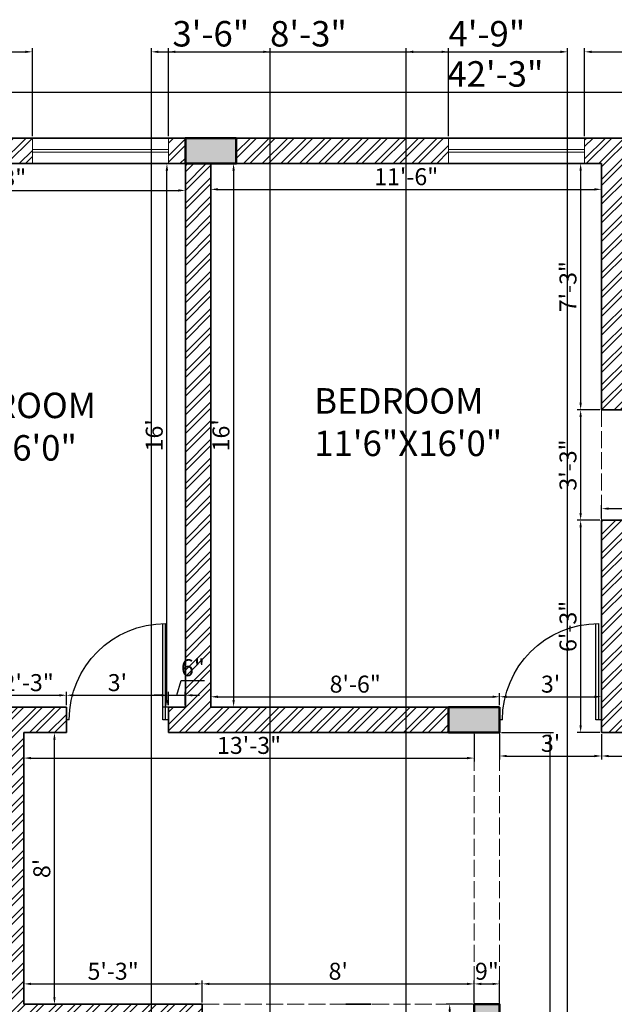
# Model space of a CAD drawing. Units: inches. Extents: x 4153 to 5577, y 785 to 1503.
# Tile 9 of 11: x 5097 to 5307, y 1138 to 1486. Entities that reach past the tile are written whole.
import ezdxf

# ---------------------------------------------------------------- set-up
doc = ezdxf.new("R2010")
doc.units = ezdxf.units.IN
doc.linetypes.add('ACAD_ISO02W100', pattern=[15, 12, -3])
for name, color, linetype, lineweight in [('A-ANNO-DIMS', 2, 'Continuous', 18), ('A-AREA-IDEN', 7, 'Continuous', 25), ('A-COLS', 7, 'Continuous', 50), ('A-DOOR', 3, 'Continuous', 25), ('A-GLAZ', 4, 'Continuous', 18), ('A-WALL', 7, 'Continuous', 35), ('A-WALL-OVHD', 7, 'ACAD_ISO02W100', 18)]:
    doc.layers.add(name, color=color, linetype=linetype, lineweight=lineweight)
doc.layers.add('A-WALL-PATT', color=251, linetype='Continuous', lineweight=13, true_color=0x636466)
doc.styles.get("Standard").update_dxf_attribs({"font": 'arial.ttf'})
doc.dimstyles.new('ISO-25', dxfattribs={"dimtxt": 9, "dimasz": 2.5, "dimexe": 1.25, "dimexo": 0.625, "dimtad": 1, "dimlunit": 3, "dimtxsty": 'Standard', "dimcen": 2.5, "dimadec": 0, "dimazin": 0, "dimtfac": 1, "dimtmove": 0, "dimatfit": 3, "dimfxl": 1, "dimarcsym": 0})

# ---------------------------------------------------------------- blocks, each defined once
blk = doc.blocks.new('D1')
for p, q in [((1, 0), (1, 34)), ((2, 0), (2, 33.99)), ((0, 0), (2, 0)), ((35, 0), (36, 0))]:
    blk.add_line(p, q)
at = {"ltscale": 0.5}
blk.add_arc((1, 0), 34, 0, 90, dxfattribs=at)
blk = doc.blocks.new('*D23')
at = {"layer": 'A-ANNO-DIMS', "color": 0, "lineweight": -2, "transparency": 16777216}
for p, q in [((5011.25, 1445.11), (5011.25, 1461.99)), ((5518.25, 1445.11), (5518.25, 1461.99)), ((5013.75, 1460.74), (5515.75, 1460.74))]:
    blk.add_line(p, q, dxfattribs=at)
at = {"layer": 'A-ANNO-DIMS', "color": 0, "transparency": 16777216}
for points in [[(5013.75, 1461.16), (5013.75, 1460.33), (5011.25, 1460.74)], [(5515.75, 1461.16), (5515.75, 1460.33), (5518.25, 1460.74)]]:
    blk.add_solid(points, dxfattribs=at)
at = {"layer": 'Defpoints', "color": 0, "transparency": 16777216}
for p in [(5518.25, 1460.74), (5011.25, 1444.49), (5518.25, 1444.49)]:
    blk.add_point(p, dxfattribs=at)
at = {"layer": 'A-ANNO-DIMS', "color": 0, "transparency": 16777216, "insert": (5264.75, 1465.97), "char_height": 9, "attachment_point": 5}
blk.add_mtext('42\'-3"', dxfattribs=at)
blk = doc.blocks.new('*D25')
at = {"layer": 'A-ANNO-DIMS', "color": 0, "lineweight": -2, "transparency": 16777216}
for p, q in [((5020.25, 1434.86), (5020.25, 1424.72)), ((5155.25, 1434.86), (5155.25, 1424.72)), ((5022.75, 1425.97), (5152.75, 1425.97))]:
    blk.add_line(p, q, dxfattribs=at)
at = {"layer": 'A-ANNO-DIMS', "color": 0, "transparency": 16777216}
for points in [[(5022.75, 1426.39), (5022.75, 1425.56), (5020.25, 1425.97)], [(5152.75, 1426.39), (5152.75, 1425.56), (5155.25, 1425.97)]]:
    blk.add_solid(points, dxfattribs=at)
at = {"layer": 'Defpoints', "color": 0, "transparency": 16777216}
for p in [(5020.25, 1435.49), (5155.25, 1435.49), (5155.25, 1425.97)]:
    blk.add_point(p, dxfattribs=at)
at = {"layer": 'A-ANNO-DIMS', "color": 0, "transparency": 16777216, "insert": (5087.75, 1429.66), "char_height": 6, "attachment_point": 5}
blk.add_mtext('11\'-3"', dxfattribs=at)
blk = doc.blocks.new('*D29')
at = {"layer": 'A-ANNO-DIMS', "color": 0, "lineweight": -2, "transparency": 16777216}
for p, q in [((5086.25, 1244.11), (5086.25, 1248.91)), ((5113.25, 1244.11), (5113.25, 1248.91)), ((5088.75, 1247.66), (5110.75, 1247.66))]:
    blk.add_line(p, q, dxfattribs=at)
at = {"layer": 'A-ANNO-DIMS', "color": 0, "transparency": 16777216}
for points in [[(5088.75, 1248.07), (5088.75, 1247.24), (5086.25, 1247.66)], [(5110.75, 1248.07), (5110.75, 1247.24), (5113.25, 1247.66)]]:
    blk.add_solid(points, dxfattribs=at)
at = {"layer": 'Defpoints', "color": 0, "transparency": 16777216}
for p in [(5113.25, 1247.66), (5086.25, 1243.49), (5113.25, 1243.49)]:
    blk.add_point(p, dxfattribs=at)
at = {"layer": 'A-ANNO-DIMS', "color": 0, "transparency": 16777216, "insert": (5099.75, 1251.35), "char_height": 6, "attachment_point": 5}
blk.add_mtext('2\'-3"', dxfattribs=at)
blk = doc.blocks.new('*D30')
at = {"layer": 'A-ANNO-DIMS', "color": 0, "lineweight": -2, "transparency": 16777216}
for p, q in [((5113.25, 1244.11), (5113.25, 1248.91)), ((5149.25, 1244.11), (5149.25, 1248.91)), ((5115.75, 1247.66), (5146.75, 1247.66))]:
    blk.add_line(p, q, dxfattribs=at)
at = {"layer": 'A-ANNO-DIMS', "color": 0, "transparency": 16777216}
for points in [[(5115.75, 1248.07), (5115.75, 1247.24), (5113.25, 1247.66)], [(5146.75, 1248.07), (5146.75, 1247.24), (5149.25, 1247.66)]]:
    blk.add_solid(points, dxfattribs=at)
at = {"layer": 'Defpoints', "color": 0, "transparency": 16777216}
for p in [(5149.25, 1247.66), (5113.25, 1243.49), (5149.25, 1243.49)]:
    blk.add_point(p, dxfattribs=at)
at = {"layer": 'A-ANNO-DIMS', "color": 0, "transparency": 16777216, "insert": (5131.25, 1251.35), "char_height": 6, "attachment_point": 5}
blk.add_mtext("3'", dxfattribs=at)
blk = doc.blocks.new('*D31')
at = {"layer": 'A-ANNO-DIMS', "color": 0, "lineweight": -2, "transparency": 16777216}
for p, q in [((5152.25, 1247.66), (5153.83, 1252.91)), ((5153.83, 1252.91), (5162.01, 1252.91)), ((5149.25, 1244.11), (5149.25, 1248.91)), ((5155.25, 1244.11), (5155.25, 1248.91)), ((5146.75, 1247.66), (5144.25, 1247.66)), ((5149.25, 1247.66), (5155.25, 1247.66)), ((5149.25, 1247.66), (5155.25, 1247.66)), ((5157.75, 1247.66), (5160.25, 1247.66))]:
    blk.add_line(p, q, dxfattribs=at)
at = {"layer": 'A-ANNO-DIMS', "color": 0, "transparency": 16777216}
for points in [[(5146.75, 1248.07), (5146.75, 1247.24), (5149.25, 1247.66)], [(5157.75, 1248.07), (5157.75, 1247.24), (5155.25, 1247.66)]]:
    blk.add_solid(points, dxfattribs=at)
at = {"layer": 'Defpoints', "color": 0, "transparency": 16777216}
for p in [(5155.25, 1247.66), (5149.25, 1243.49), (5155.25, 1243.49)]:
    blk.add_point(p, dxfattribs=at)
at = {"layer": 'A-ANNO-DIMS', "color": 0, "transparency": 16777216, "insert": (5157.92, 1256.6), "char_height": 6, "attachment_point": 5}
blk.add_mtext('6"', dxfattribs=at)
blk = doc.blocks.new('*D32')
at = {"layer": 'A-ANNO-DIMS', "color": 0, "lineweight": -2, "transparency": 16777216}
for p, q in [((5154.63, 1435.49), (5147.49, 1435.49)), ((5148.74, 1245.99), (5148.74, 1432.99)), ((5154.63, 1243.49), (5147.49, 1243.49))]:
    blk.add_line(p, q, dxfattribs=at)
at = {"layer": 'A-ANNO-DIMS', "color": 0, "transparency": 16777216}
for points in [[(5148.32, 1432.99), (5149.16, 1432.99), (5148.74, 1435.49)], [(5148.32, 1245.99), (5149.16, 1245.99), (5148.74, 1243.49)]]:
    blk.add_solid(points, dxfattribs=at)
at = {"layer": 'Defpoints', "color": 0, "transparency": 16777216}
for p in [(5148.74, 1435.49), (5155.25, 1435.49), (5155.25, 1243.49)]:
    blk.add_point(p, dxfattribs=at)
at = {"layer": 'A-ANNO-DIMS', "color": 0, "transparency": 16777216, "insert": (5145.05, 1339.49), "char_height": 6, "attachment_point": 5, "rotation": 90}
blk.add_mtext("16'", dxfattribs=at)
blk = doc.blocks.new('*D33')
at = {"layer": 'A-ANNO-DIMS', "color": 0, "lineweight": -2, "transparency": 16777216}
for p, q in [((5164.25, 1434.86), (5164.25, 1425.11)), ((5302.25, 1434.86), (5302.25, 1425.11)), ((5166.75, 1426.36), (5299.75, 1426.36))]:
    blk.add_line(p, q, dxfattribs=at)
at = {"layer": 'A-ANNO-DIMS', "color": 0, "transparency": 16777216}
for points in [[(5166.75, 1426.78), (5166.75, 1425.94), (5164.25, 1426.36)], [(5299.75, 1426.78), (5299.75, 1425.94), (5302.25, 1426.36)]]:
    blk.add_solid(points, dxfattribs=at)
at = {"layer": 'Defpoints', "color": 0, "transparency": 16777216}
for p in [(5164.25, 1435.49), (5302.25, 1435.49), (5302.25, 1426.36)]:
    blk.add_point(p, dxfattribs=at)
at = {"layer": 'A-ANNO-DIMS', "color": 0, "transparency": 16777216, "insert": (5233.25, 1430.05), "char_height": 6, "attachment_point": 5}
blk.add_mtext('11\'-6"', dxfattribs=at)
blk = doc.blocks.new('*D34')
at = {"layer": 'A-ANNO-DIMS', "color": 0, "lineweight": -2, "transparency": 16777216}
for p, q in [((5164.88, 1435.49), (5173.55, 1435.49)), ((5172.3, 1432.99), (5172.3, 1245.99)), ((5164.88, 1243.49), (5173.55, 1243.49))]:
    blk.add_line(p, q, dxfattribs=at)
at = {"layer": 'A-ANNO-DIMS', "color": 0, "transparency": 16777216}
for points in [[(5171.88, 1432.99), (5172.72, 1432.99), (5172.3, 1435.49)], [(5171.88, 1245.99), (5172.72, 1245.99), (5172.3, 1243.49)]]:
    blk.add_solid(points, dxfattribs=at)
at = {"layer": 'Defpoints', "color": 0, "transparency": 16777216}
for p in [(5164.25, 1435.49), (5164.25, 1243.49), (5172.3, 1243.49)]:
    blk.add_point(p, dxfattribs=at)
at = {"layer": 'A-ANNO-DIMS', "color": 0, "transparency": 16777216, "insert": (5168.61, 1339.49), "char_height": 6, "attachment_point": 5, "rotation": 90}
blk.add_mtext("16'", dxfattribs=at)
blk = doc.blocks.new('*D35')
at = {"layer": 'A-ANNO-DIMS', "color": 0, "lineweight": -2, "transparency": 16777216}
for p, q in [((5164.25, 1244.11), (5164.25, 1248.37)), ((5166.75, 1247.12), (5263.75, 1247.12)), ((5266.25, 1244.11), (5266.25, 1248.37))]:
    blk.add_line(p, q, dxfattribs=at)
at = {"layer": 'A-ANNO-DIMS', "color": 0, "transparency": 16777216}
for points in [[(5166.75, 1247.54), (5166.75, 1246.7), (5164.25, 1247.12)], [(5263.75, 1247.54), (5263.75, 1246.7), (5266.25, 1247.12)]]:
    blk.add_solid(points, dxfattribs=at)
at = {"layer": 'Defpoints', "color": 0, "transparency": 16777216}
for p in [(5266.25, 1247.12), (5164.25, 1243.49), (5266.25, 1243.49)]:
    blk.add_point(p, dxfattribs=at)
at = {"layer": 'A-ANNO-DIMS', "color": 0, "transparency": 16777216, "insert": (5215.25, 1250.81), "char_height": 6, "attachment_point": 5}
blk.add_mtext('8\'-6"', dxfattribs=at)
blk = doc.blocks.new('*D36')
at = {"layer": 'A-ANNO-DIMS', "color": 0, "lineweight": -2, "transparency": 16777216}
for p, q in [((5266.25, 1244.11), (5266.25, 1248.37)), ((5268.75, 1247.12), (5299.75, 1247.12)), ((5302.25, 1247.75), (5302.25, 1248.37))]:
    blk.add_line(p, q, dxfattribs=at)
at = {"layer": 'A-ANNO-DIMS', "color": 0, "transparency": 16777216}
for points in [[(5268.75, 1247.54), (5268.75, 1246.7), (5266.25, 1247.12)], [(5299.75, 1247.54), (5299.75, 1246.7), (5302.25, 1247.12)]]:
    blk.add_solid(points, dxfattribs=at)
at = {"layer": 'Defpoints', "color": 0, "transparency": 16777216}
for p in [(5302.25, 1247.12), (5302.25, 1247.12), (5266.25, 1243.49)]:
    blk.add_point(p, dxfattribs=at)
at = {"layer": 'A-ANNO-DIMS', "color": 0, "transparency": 16777216, "insert": (5284.25, 1250.81), "char_height": 6, "attachment_point": 5}
blk.add_mtext("3'", dxfattribs=at)
blk = doc.blocks.new('*D37')
at = {"layer": 'A-ANNO-DIMS', "color": 0, "lineweight": -2, "transparency": 16777216}
for p, q in [((5301.63, 1435.49), (5293.61, 1435.49)), ((5294.86, 1432.99), (5294.86, 1350.99)), ((5301.63, 1348.49), (5293.61, 1348.49))]:
    blk.add_line(p, q, dxfattribs=at)
at = {"layer": 'A-ANNO-DIMS', "color": 0, "transparency": 16777216}
for points in [[(5294.45, 1432.99), (5295.28, 1432.99), (5294.86, 1435.49)], [(5294.45, 1350.99), (5295.28, 1350.99), (5294.86, 1348.49)]]:
    blk.add_solid(points, dxfattribs=at)
at = {"layer": 'Defpoints', "color": 0, "transparency": 16777216}
for p in [(5302.25, 1435.49), (5294.86, 1348.49), (5302.25, 1348.49)]:
    blk.add_point(p, dxfattribs=at)
at = {"layer": 'A-ANNO-DIMS', "color": 0, "transparency": 16777216, "insert": (5291.17, 1391.99), "char_height": 6, "attachment_point": 5, "rotation": 90}
blk.add_mtext('7\'-3"', dxfattribs=at)
blk = doc.blocks.new('*D38')
at = {"layer": 'A-ANNO-DIMS', "color": 0, "lineweight": -2, "transparency": 16777216}
for p, q in [((5301.63, 1348.49), (5293.61, 1348.49)), ((5294.86, 1345.99), (5294.86, 1311.99)), ((5301.63, 1309.49), (5293.61, 1309.49))]:
    blk.add_line(p, q, dxfattribs=at)
at = {"layer": 'A-ANNO-DIMS', "color": 0, "transparency": 16777216}
for points in [[(5294.45, 1345.99), (5295.28, 1345.99), (5294.86, 1348.49)], [(5294.45, 1311.99), (5295.28, 1311.99), (5294.86, 1309.49)]]:
    blk.add_solid(points, dxfattribs=at)
at = {"layer": 'Defpoints', "color": 0, "transparency": 16777216}
for p in [(5302.25, 1348.49), (5294.86, 1309.49), (5302.25, 1309.49)]:
    blk.add_point(p, dxfattribs=at)
at = {"layer": 'A-ANNO-DIMS', "color": 0, "transparency": 16777216, "insert": (5291.17, 1328.99), "char_height": 6, "attachment_point": 5, "rotation": 90}
blk.add_mtext('3\'-3"', dxfattribs=at)
blk = doc.blocks.new('*D39')
at = {"layer": 'A-ANNO-DIMS', "color": 0, "lineweight": -2, "transparency": 16777216}
for p, q in [((5301.63, 1309.49), (5293.61, 1309.49)), ((5294.86, 1306.99), (5294.86, 1236.99)), ((5301.63, 1234.49), (5293.61, 1234.49))]:
    blk.add_line(p, q, dxfattribs=at)
at = {"layer": 'A-ANNO-DIMS', "color": 0, "transparency": 16777216}
for points in [[(5294.45, 1306.99), (5295.28, 1306.99), (5294.86, 1309.49)], [(5294.45, 1236.99), (5295.28, 1236.99), (5294.86, 1234.49)]]:
    blk.add_solid(points, dxfattribs=at)
at = {"layer": 'Defpoints', "color": 0, "transparency": 16777216}
for p in [(5302.25, 1309.49), (5294.86, 1234.49), (5302.25, 1234.49)]:
    blk.add_point(p, dxfattribs=at)
at = {"layer": 'A-ANNO-DIMS', "color": 0, "transparency": 16777216, "insert": (5291.17, 1271.99), "char_height": 6, "attachment_point": 5, "rotation": 90}
blk.add_mtext('6\'-3"', dxfattribs=at)
blk = doc.blocks.new('*D40')
at = {"layer": 'A-ANNO-DIMS', "color": 0, "lineweight": -2, "transparency": 16777216}
for p, q in [((5098.25, 1233.86), (5098.25, 1224.22)), ((5257.25, 1233.86), (5257.25, 1224.22)), ((5100.75, 1225.47), (5254.75, 1225.47))]:
    blk.add_line(p, q, dxfattribs=at)
at = {"layer": 'A-ANNO-DIMS', "color": 0, "transparency": 16777216}
for points in [[(5100.75, 1225.88), (5100.75, 1225.05), (5098.25, 1225.47)], [(5254.75, 1225.88), (5254.75, 1225.05), (5257.25, 1225.47)]]:
    blk.add_solid(points, dxfattribs=at)
at = {"layer": 'Defpoints', "color": 0, "transparency": 16777216}
for p in [(5098.25, 1234.49), (5257.25, 1234.49), (5257.25, 1225.47)]:
    blk.add_point(p, dxfattribs=at)
at = {"layer": 'A-ANNO-DIMS', "color": 0, "transparency": 16777216, "insert": (5177.75, 1229.16), "char_height": 6, "attachment_point": 5}
blk.add_mtext('13\'-3"', dxfattribs=at)
blk = doc.blocks.new('*D53')
at = {"layer": 'A-ANNO-DIMS', "color": 0, "lineweight": -2, "transparency": 16777216}
for p, q in [((5256.63, 1138.49), (5247.37, 1138.49)), ((5248.62, 1002.99), (5248.62, 1135.99)), ((5256.63, 1000.49), (5247.37, 1000.49))]:
    blk.add_line(p, q, dxfattribs=at)
at = {"layer": 'A-ANNO-DIMS', "color": 0, "transparency": 16777216}
for points in [[(5248.2, 1135.99), (5249.04, 1135.99), (5248.62, 1138.49)], [(5248.2, 1002.99), (5249.04, 1002.99), (5248.62, 1000.49)]]:
    blk.add_solid(points, dxfattribs=at)
at = {"layer": 'Defpoints', "color": 0, "transparency": 16777216}
for p in [(5248.62, 1138.49), (5257.25, 1138.49), (5257.25, 1000.49)]:
    blk.add_point(p, dxfattribs=at)
at = {"layer": 'A-ANNO-DIMS', "color": 0, "transparency": 16777216, "insert": (5244.93, 1069.49), "char_height": 6, "attachment_point": 5, "rotation": 90}
blk.add_mtext('11\'-6"', dxfattribs=at)
blk = doc.blocks.new('*D54')
at = {"layer": 'A-ANNO-DIMS', "color": 0, "lineweight": -2, "transparency": 16777216}
for p, q in [((5266.88, 1234.49), (5285.33, 1234.49)), ((5284.08, 1002.99), (5284.08, 1231.99)), ((5266.88, 1000.49), (5285.33, 1000.49))]:
    blk.add_line(p, q, dxfattribs=at)
at = {"layer": 'A-ANNO-DIMS', "color": 0, "transparency": 16777216}
for points in [[(5283.66, 1231.99), (5284.49, 1231.99), (5284.08, 1234.49)], [(5283.66, 1002.99), (5284.49, 1002.99), (5284.08, 1000.49)]]:
    blk.add_solid(points, dxfattribs=at)
at = {"layer": 'Defpoints', "color": 0, "transparency": 16777216}
for p in [(5266.25, 1234.49), (5284.08, 1234.49), (5266.25, 1000.49)]:
    blk.add_point(p, dxfattribs=at)
at = {"layer": 'A-ANNO-DIMS', "color": 0, "transparency": 16777216, "insert": (5280.39, 1117.49), "char_height": 6, "attachment_point": 5, "rotation": 90}
blk.add_mtext('19\'-6"', dxfattribs=at)
blk = doc.blocks.new('*D59')
at = {"layer": 'A-ANNO-DIMS', "color": 0, "lineweight": -2, "transparency": 16777216}
for p, q in [((5266.25, 1233.86), (5266.25, 1224.95)), ((5302.25, 1233.86), (5302.25, 1224.95)), ((5268.75, 1226.2), (5299.75, 1226.2))]:
    blk.add_line(p, q, dxfattribs=at)
at = {"layer": 'A-ANNO-DIMS', "color": 0, "transparency": 16777216}
for points in [[(5268.75, 1226.62), (5268.75, 1225.78), (5266.25, 1226.2)], [(5299.75, 1226.62), (5299.75, 1225.78), (5302.25, 1226.2)]]:
    blk.add_solid(points, dxfattribs=at)
at = {"layer": 'Defpoints', "color": 0, "transparency": 16777216}
for p in [(5266.25, 1234.49), (5302.25, 1234.49), (5302.25, 1226.2)]:
    blk.add_point(p, dxfattribs=at)
at = {"layer": 'A-ANNO-DIMS', "color": 0, "transparency": 16777216, "insert": (5284.25, 1229.89), "char_height": 6, "attachment_point": 5}
blk.add_mtext("3'", dxfattribs=at)
blk = doc.blocks.new('*D60')
at = {"layer": 'A-ANNO-DIMS', "color": 0, "lineweight": -2, "transparency": 16777216}
for p, q in [((5302.25, 1233.86), (5302.25, 1224.95)), ((5321.75, 1233.86), (5321.75, 1224.95)), ((5304.75, 1226.2), (5319.25, 1226.2)), ((5312, 1226.2), (5315.42, 1214.82)), ((5315.42, 1214.82), (5339.04, 1214.82))]:
    blk.add_line(p, q, dxfattribs=at)
at = {"layer": 'A-ANNO-DIMS', "color": 0, "transparency": 16777216}
for points in [[(5304.75, 1226.62), (5304.75, 1225.78), (5302.25, 1226.2)], [(5319.25, 1226.62), (5319.25, 1225.78), (5321.75, 1226.2)]]:
    blk.add_solid(points, dxfattribs=at)
at = {"layer": 'Defpoints', "color": 0, "transparency": 16777216}
for p in [(5302.25, 1234.49), (5321.75, 1234.49), (5321.75, 1226.2)]:
    blk.add_point(p, dxfattribs=at)
at = {"layer": 'A-ANNO-DIMS', "color": 0, "transparency": 16777216, "insert": (5327.23, 1218.51), "char_height": 6, "attachment_point": 5}
blk.add_mtext('1\'-7.5"', dxfattribs=at)
blk = doc.blocks.new('*D74')
at = {"layer": 'A-ANNO-DIMS', "color": 0, "lineweight": -2, "transparency": 16777216}
for p, q in [((5302.25, 1310.11), (5302.25, 1314.82)), ((5368.25, 1310.11), (5368.25, 1314.82)), ((5304.75, 1313.57), (5365.75, 1313.57))]:
    blk.add_line(p, q, dxfattribs=at)
at = {"layer": 'A-ANNO-DIMS', "color": 0, "transparency": 16777216}
for points in [[(5304.75, 1313.99), (5304.75, 1313.15), (5302.25, 1313.57)], [(5365.75, 1313.99), (5365.75, 1313.15), (5368.25, 1313.57)]]:
    blk.add_solid(points, dxfattribs=at)
at = {"layer": 'Defpoints', "color": 0, "transparency": 16777216}
for p in [(5368.25, 1313.57), (5302.25, 1309.49), (5368.25, 1309.49)]:
    blk.add_point(p, dxfattribs=at)
at = {"layer": 'A-ANNO-DIMS', "color": 0, "transparency": 16777216, "insert": (5335.25, 1317.26), "char_height": 6, "attachment_point": 5}
blk.add_mtext('5\'-6"', dxfattribs=at)
blk = doc.blocks.new('*D83')
at = {"layer": 'A-ANNO-DIMS', "color": 0, "lineweight": -2, "transparency": 16777216}
for p, q in [((5098.88, 1234.49), (5110.28, 1234.49)), ((5109.03, 1140.99), (5109.03, 1231.99)), ((5098.88, 1138.49), (5110.28, 1138.49))]:
    blk.add_line(p, q, dxfattribs=at)
at = {"layer": 'A-ANNO-DIMS', "color": 0, "transparency": 16777216}
for points in [[(5108.61, 1231.99), (5109.44, 1231.99), (5109.03, 1234.49)], [(5108.61, 1140.99), (5109.44, 1140.99), (5109.03, 1138.49)]]:
    blk.add_solid(points, dxfattribs=at)
at = {"layer": 'Defpoints', "color": 0, "transparency": 16777216}
for p in [(5098.25, 1234.49), (5109.03, 1234.49), (5098.25, 1138.49)]:
    blk.add_point(p, dxfattribs=at)
at = {"layer": 'A-ANNO-DIMS', "color": 0, "transparency": 16777216, "insert": (5105.34, 1186.49), "char_height": 6, "attachment_point": 5, "rotation": 90}
blk.add_mtext("8'", dxfattribs=at)
blk = doc.blocks.new('*D84')
at = {"layer": 'A-ANNO-DIMS', "color": 0, "lineweight": -2, "transparency": 16777216}
for p, q in [((5098.25, 1139.11), (5098.25, 1146.95)), ((5100.75, 1145.7), (5158.75, 1145.7)), ((5161.25, 1139.11), (5161.25, 1146.95))]:
    blk.add_line(p, q, dxfattribs=at)
at = {"layer": 'A-ANNO-DIMS', "color": 0, "transparency": 16777216}
for points in [[(5100.75, 1146.11), (5100.75, 1145.28), (5098.25, 1145.7)], [(5158.75, 1146.11), (5158.75, 1145.28), (5161.25, 1145.7)]]:
    blk.add_solid(points, dxfattribs=at)
at = {"layer": 'Defpoints', "color": 0, "transparency": 16777216}
for p in [(5161.25, 1145.7), (5098.25, 1138.49), (5161.25, 1138.49)]:
    blk.add_point(p, dxfattribs=at)
at = {"layer": 'A-ANNO-DIMS', "color": 0, "transparency": 16777216, "insert": (5129.75, 1149.39), "char_height": 6, "attachment_point": 5}
blk.add_mtext('5\'-3"', dxfattribs=at)
blk = doc.blocks.new('*D85')
at = {"layer": 'A-ANNO-DIMS', "color": 0, "lineweight": -2, "transparency": 16777216}
for p, q in [((5161.25, 1139.11), (5161.25, 1146.95)), ((5163.75, 1145.7), (5254.75, 1145.7)), ((5257.25, 1139.11), (5257.25, 1146.95))]:
    blk.add_line(p, q, dxfattribs=at)
at = {"layer": 'A-ANNO-DIMS', "color": 0, "transparency": 16777216}
for points in [[(5163.75, 1146.11), (5163.75, 1145.28), (5161.25, 1145.7)], [(5254.75, 1146.11), (5254.75, 1145.28), (5257.25, 1145.7)]]:
    blk.add_solid(points, dxfattribs=at)
at = {"layer": 'Defpoints', "color": 0, "transparency": 16777216}
for p in [(5257.25, 1145.7), (5161.25, 1138.49), (5257.25, 1138.49)]:
    blk.add_point(p, dxfattribs=at)
at = {"layer": 'A-ANNO-DIMS', "color": 0, "transparency": 16777216, "insert": (5209.25, 1149.39), "char_height": 6, "attachment_point": 5}
blk.add_mtext("8'", dxfattribs=at)
blk = doc.blocks.new('*D86')
at = {"layer": 'A-ANNO-DIMS', "color": 0, "lineweight": -2, "transparency": 16777216}
for p, q in [((5257.25, 1139.11), (5257.25, 1146.95)), ((5259.75, 1145.7), (5263.75, 1145.7)), ((5266.25, 1139.11), (5266.25, 1146.95))]:
    blk.add_line(p, q, dxfattribs=at)
at = {"layer": 'A-ANNO-DIMS', "color": 0, "transparency": 16777216}
for points in [[(5259.75, 1146.11), (5259.75, 1145.28), (5257.25, 1145.7)], [(5263.75, 1146.11), (5263.75, 1145.28), (5266.25, 1145.7)]]:
    blk.add_solid(points, dxfattribs=at)
at = {"layer": 'Defpoints', "color": 0, "transparency": 16777216}
for p in [(5266.25, 1145.7), (5257.25, 1138.49), (5266.25, 1138.49)]:
    blk.add_point(p, dxfattribs=at)
at = {"layer": 'A-ANNO-DIMS', "color": 0, "transparency": 16777216, "insert": (5261.75, 1149.39), "char_height": 6, "attachment_point": 5}
blk.add_mtext('9"', dxfattribs=at)
blk = doc.blocks.new('WINDOW-48IN')
for p, q in [((0, 9), (0, 0)), ((48, 9), (48, 0)), ((0, 5), (48, 5)), ((0, 4), (48, 4))]:
    blk.add_line(p, q)
blk = doc.blocks.new('COL-9X18IN')
at = {"transparency": 33554687}
h = blk.add_hatch(color=256, dxfattribs=at)
h.dxf.hatch_style = 1
h.paths.add_polyline_path([(9, 18), (0, 18), (0, 0), (9, 0)])
blk.add_lwpolyline([(0, 18), (9, 18), (9, 0), (0, 0)], close=True)
blk = doc.blocks.new('*D146')
at = {"layer": 'A-ANNO-DIMS', "color": 0, "lineweight": -2, "transparency": 16777216}
for p, q in [((5011.25, 1445.11), (5011.25, 1476.19)), ((5013.75, 1474.94), (5098.75, 1474.94)), ((5101.25, 1445.11), (5101.25, 1476.19))]:
    blk.add_line(p, q, dxfattribs=at)
at = {"layer": 'A-ANNO-DIMS', "color": 0, "transparency": 16777216}
for points in [[(5013.75, 1475.36), (5013.75, 1474.52), (5011.25, 1474.94)], [(5098.75, 1475.36), (5098.75, 1474.52), (5101.25, 1474.94)]]:
    blk.add_solid(points, dxfattribs=at)
at = {"layer": 'Defpoints', "color": 0, "transparency": 16777216}
for p in [(5101.25, 1474.94), (5011.25, 1444.49), (5101.25, 1444.49)]:
    blk.add_point(p, dxfattribs=at)
at = {"layer": 'A-ANNO-DIMS', "color": 0, "transparency": 16777216, "insert": (5056.25, 1480.16), "char_height": 9, "attachment_point": 5}
blk.add_mtext('7\'-6"', dxfattribs=at)
blk = doc.blocks.new('*D147')
at = {"layer": 'A-ANNO-DIMS', "color": 0, "lineweight": -2, "transparency": 16777216}
for p, q in [((5149.25, 1445.11), (5149.25, 1476.19)), ((5151.75, 1474.94), (5245.75, 1474.94)), ((5248.25, 1445.11), (5248.25, 1476.19))]:
    blk.add_line(p, q, dxfattribs=at)
at = {"layer": 'A-ANNO-DIMS', "color": 0, "transparency": 16777216}
for points in [[(5151.75, 1475.36), (5151.75, 1474.52), (5149.25, 1474.94)], [(5245.75, 1475.36), (5245.75, 1474.52), (5248.25, 1474.94)]]:
    blk.add_solid(points, dxfattribs=at)
at = {"layer": 'Defpoints', "color": 0, "transparency": 16777216}
for p in [(5248.25, 1474.94), (5149.25, 1444.49), (5248.25, 1444.49)]:
    blk.add_point(p, dxfattribs=at)
at = {"layer": 'A-ANNO-DIMS', "color": 0, "transparency": 16777216, "insert": (5198.75, 1480.16), "char_height": 9, "attachment_point": 5}
blk.add_mtext('8\'-3"', dxfattribs=at)
blk = doc.blocks.new('*D148')
at = {"layer": 'A-ANNO-DIMS', "color": 0, "lineweight": -2, "transparency": 16777216}
for p, q in [((5296.25, 1445.11), (5296.25, 1476.19)), ((5298.75, 1474.94), (5311.75, 1474.94)), ((5314.25, 1445.11), (5314.25, 1476.19)), ((5314.25, 1474.94), (5341.08, 1474.94))]:
    blk.add_line(p, q, dxfattribs=at)
at = {"layer": 'A-ANNO-DIMS', "color": 0, "transparency": 16777216}
for points in [[(5298.75, 1475.36), (5298.75, 1474.52), (5296.25, 1474.94)], [(5311.75, 1475.36), (5311.75, 1474.52), (5314.25, 1474.94)]]:
    blk.add_solid(points, dxfattribs=at)
at = {"layer": 'Defpoints', "color": 0, "transparency": 16777216}
for p in [(5314.25, 1474.94), (5296.25, 1444.49), (5314.25, 1444.49)]:
    blk.add_point(p, dxfattribs=at)
at = {"layer": 'A-ANNO-DIMS', "color": 0, "transparency": 16777216, "insert": (5328.92, 1480.16), "char_height": 9, "attachment_point": 5}
blk.add_mtext('1\'-6"', dxfattribs=at)
blk = doc.blocks.new('*D157')
at = {"layer": 'A-ANNO-DIMS', "color": 0, "lineweight": -2, "transparency": 16777216}
for p, q in [((5143.25, 1001.11), (5143.25, 1476.19)), ((5145.75, 1474.94), (5182.75, 1474.94)), ((5185.25, 1001.11), (5185.25, 1476.19))]:
    blk.add_line(p, q, dxfattribs=at)
at = {"layer": 'A-ANNO-DIMS', "color": 0, "transparency": 16777216}
for points in [[(5145.75, 1475.36), (5145.75, 1474.52), (5143.25, 1474.94)], [(5182.75, 1475.36), (5182.75, 1474.52), (5185.25, 1474.94)]]:
    blk.add_solid(points, dxfattribs=at)
at = {"layer": 'Defpoints', "color": 0, "transparency": 16777216}
for p in [(5185.25, 1474.94), (5143.25, 1000.49), (5185.25, 1000.49)]:
    blk.add_point(p, dxfattribs=at)
at = {"layer": 'A-ANNO-DIMS', "color": 0, "transparency": 16777216, "insert": (5164.25, 1480.16), "char_height": 9, "attachment_point": 5}
blk.add_mtext('3\'-6"', dxfattribs=at)
blk = doc.blocks.new('*D158')
at = {"layer": 'A-ANNO-DIMS', "color": 0, "lineweight": -2, "transparency": 16777216}
for p, q in [((5233.25, 1001.11), (5233.25, 1476.19)), ((5235.75, 1474.94), (5287.75, 1474.94)), ((5290.25, 1001.11), (5290.25, 1476.19))]:
    blk.add_line(p, q, dxfattribs=at)
at = {"layer": 'A-ANNO-DIMS', "color": 0, "transparency": 16777216}
for points in [[(5235.75, 1475.36), (5235.75, 1474.52), (5233.25, 1474.94)], [(5287.75, 1475.36), (5287.75, 1474.52), (5290.25, 1474.94)]]:
    blk.add_solid(points, dxfattribs=at)
at = {"layer": 'Defpoints', "color": 0, "transparency": 16777216}
for p in [(5290.25, 1474.94), (5233.25, 1000.49), (5290.25, 1000.49)]:
    blk.add_point(p, dxfattribs=at)
at = {"layer": 'A-ANNO-DIMS', "color": 0, "transparency": 16777216, "insert": (5261.75, 1480.16), "char_height": 9, "attachment_point": 5}
blk.add_mtext('4\'-9"', dxfattribs=at)

msp = doc.modelspace()

# ---------------------------------------------------------------- hatches: boundary and pattern name
at = {"layer": 'A-WALL-PATT', "transparency": 33554687}
h = msp.add_hatch(dxfattribs=at)
h.set_pattern_fill('ANSI32', color=256, scale=0.5)
h.paths.add_polyline_path([(5155.254, 1444.488), (5149.254, 1444.488), (5149.254, 1435.488), (5155.254, 1435.488)])
h.paths.add_polyline_path([(4338.927, 1444.488), (4332.927, 1444.488), (4332.927, 1435.488), (4338.927, 1435.488)])
h = msp.add_hatch(dxfattribs=at)
h.set_pattern_fill('ANSI32', color=256, scale=0.49)
h.set_pattern_definition([(45, (816.3263, 0), (-3.300244, 3.300244), []), (45, (818.5265, 0), (-3.300244, 3.300244), [])])
h.paths.add_polyline_path([(5011.254, 1088.988), (5020.254, 1088.988), (5020.254, 1129.488), (5155.254, 1129.488), (5155.254, 1105.488), (5161.254, 1105.488), (5161.254, 1138.488), (5098.254, 1138.488), (5098.254, 1234.488), (5113.254, 1234.488), (5113.254, 1243.488), (5086.254, 1243.488), (5086.254, 1234.488), (5092.254, 1234.488), (5092.254, 1138.488), (5020.254, 1138.488), (5020.254, 1168.488), (5011.254, 1168.488)])
h.paths.add_polyline_path([(5011.254, 1009.488), (5020.254, 1009.488), (5020.254, 1040.988), (5011.254, 1040.988)])
h.paths.add_polyline_path([(5095.254, 991.488), (5095.254, 1000.488), (5020.254, 1000.488), (5020.254, 991.488)])
h.paths.add_polyline_path([(5011.254, 910.488), (5020.254, 910.488), (5020.254, 991.488), (5011.254, 991.488)])
h.paths.add_polyline_path([(5152.254, 901.488), (5152.254, 907.488), (5020.254, 907.488), (5020.254, 901.488)])
h.paths.add_polyline_path([(5161.254, 1057.488), (5155.254, 1057.488), (5155.254, 1000.488), (5161.254, 1000.488)])
h.paths.add_polyline_path([(5143.254, 991.488), (5152.254, 991.488), (5152.254, 1000.488), (5143.254, 1000.488)])
h.paths.add_polyline_path([(5161.254, 1000.488), (5161.254, 991.488), (5185.254, 991.488), (5185.254, 1000.488)])
h.paths.add_polyline_path([(5257.254, 991.488), (5257.254, 1000.488), (5233.254, 1000.488), (5233.254, 991.488)])
h.paths.add_polyline_path([(5266.254, 1120.488), (5257.254, 1120.488), (5257.254, 1000.488), (5266.254, 1000.488)])
h.paths.add_polyline_path([(5290.254, 991.488), (5290.254, 1000.488), (5275.254, 1000.488), (5275.254, 991.488)])
h.paths.add_polyline_path([(5362.254, 1000.488), (5362.254, 991.488), (5455.254, 991.488), (5455.254, 1000.488)])
h.paths.add_polyline_path([(5509.254, 1009.488), (5518.254, 1009.488), (5518.254, 1036.488), (5509.254, 1036.488)])
h.paths.add_polyline_path([(5503.254, 1000.488), (5503.254, 991.488), (5509.254, 991.488), (5509.254, 1000.488)])
h.paths.add_polyline_path([(5518.254, 1132.488), (5509.254, 1132.488), (5509.254, 1108.488), (5518.254, 1108.488)])
h.paths.add_polyline_path([(5509.254, 1204.488), (5518.254, 1204.488), (5518.254, 1225.488), (5509.254, 1225.488)])
h.paths.add_polyline_path([(5467.254, 1234.488), (5467.254, 1243.488), (5377.254, 1243.488), (5377.254, 1265.228), (5377.254, 1381.488), (5467.254, 1381.488), (5467.254, 1393.488), (5461.254, 1393.488), (5461.254, 1387.488), (5377.254, 1387.488), (5377.254, 1435.488), (5368.254, 1435.488), (5368.254, 1354.488), (5347.254, 1354.488), (5347.254, 1348.488), (5368.254, 1348.488), (5368.254, 1309.488), (5302.254, 1309.488), (5302.254, 1234.488), (5321.754, 1234.488), (5321.754, 1243.488), (5311.254, 1243.488), (5311.254, 1303.488), (5368.254, 1303.488), (5368.254, 1243.488), (5357.754, 1243.488), (5357.754, 1234.488)])
h.paths.add_polyline_path([(5509.254, 1357.488), (5518.254, 1357.488), (5518.254, 1426.488), (5509.254, 1426.488)])
h.paths.add_polyline_path([(5509.254, 1243.488), (5518.254, 1243.488), (5518.254, 1309.488), (5509.254, 1309.488)])
h.paths.add_polyline_path([(5509.254, 1435.488), (5509.254, 1444.488), (5425.254, 1444.488), (5425.254, 1435.488), (5461.254, 1435.488), (5461.254, 1423.488), (5467.254, 1423.488), (5467.254, 1435.488)])
h.paths.add_polyline_path([(5302.254, 1435.488), (5302.254, 1348.488), (5317.254, 1348.488), (5317.254, 1354.488), (5311.254, 1354.488), (5311.254, 1435.488), (5314.254, 1435.488), (5314.254, 1444.488), (5296.254, 1444.488), (5296.254, 1435.488)])
h.paths.add_polyline_path([(5368.254, 1444.488), (5362.254, 1444.488), (5362.254, 1435.488), (5368.254, 1435.488)])
h.paths.add_polyline_path([(5389.254, 1444.488), (5386.254, 1444.488), (5386.254, 1435.488), (5389.254, 1435.488)])
h.paths.add_polyline_path([(5248.254, 1435.488), (5248.254, 1444.488), (5173.254, 1444.488), (5173.254, 1435.488)])
h.paths.add_polyline_path([(5101.254, 1435.488), (5101.254, 1444.488), (5020.254, 1444.488), (5020.254, 1435.488)])
h.paths.add_polyline_path([(5011.254, 1293.488), (5020.254, 1293.488), (5020.254, 1295.242), (5020.254, 1426.488), (5011.254, 1426.488)])
h.paths.add_polyline_path([(5155.254, 1243.488), (5149.254, 1243.488), (5149.254, 1234.488), (5248.254, 1234.488), (5248.254, 1243.488), (5164.254, 1243.488), (5164.254, 1435.488), (5155.254, 1435.488)])
h.paths.add_polyline_path([(5020.254, 1243.488), (5020.254, 1234.488), (5056.254, 1234.488), (5056.254, 1243.488)], flags=17)
h.paths.add_polyline_path([(5020.254, 1225.488), (5011.254, 1225.488), (5011.254, 1198.488), (5020.254, 1198.488)], flags=17)

# ---------------------------------------------------------------- linework, layer by layer
at = {"layer": 'A-WALL'}
for p, q in [((5011.254, 1444.488), (5518.254, 1444.488)), ((5020.254, 1435.488), (5155.254, 1435.488)), ((5155.254, 1243.488), (5155.254, 1435.488)), ((5164.254, 1435.488), (5302.254, 1435.488)), ((5164.254, 1243.488), (5164.254, 1435.488)), ((5302.254, 1348.488), (5302.254, 1435.488)), ((5302.254, 1348.488), (5317.254, 1348.488)), ((5302.254, 1309.488), (5368.254, 1309.488)), ((5302.254, 1234.488), (5302.254, 1309.488)), ((5086.254, 1243.488), (5113.254, 1243.488)), ((5113.254, 1234.488), (5113.254, 1243.488)), ((5149.254, 1243.488), (5155.254, 1243.488)), ((5149.254, 1234.488), (5149.254, 1243.488)), ((5164.254, 1243.488), (5266.254, 1243.488)), ((5266.254, 1234.488), (5266.254, 1243.488)), ((5098.254, 1234.488), (5113.254, 1234.488)), ((5098.254, 1138.488), (5098.254, 1234.488)), ((5149.254, 1234.488), (5266.254, 1234.488)), ((5302.254, 1234.488), (5321.754, 1234.488)), ((5098.254, 1138.488), (5161.254, 1138.488)), ((5161.254, 1105.488), (5161.254, 1138.488)), ((5211.9, 1138.488), (5220.9, 1138.488)), ((5257.254, 1138.488), (5266.254, 1138.488)), ((5257.254, 1000.488), (5257.254, 1138.488)), ((5266.254, 1000.488), (5266.254, 1138.488))]:
    msp.add_line(p, q, dxfattribs=at)
at = {"layer": 'A-WALL-OVHD', "ltscale": 0.5}
for p, q in [((5302.254, 1348.488), (5302.254, 1309.488)), ((5257.254, 1138.488), (5257.254, 1234.488)), ((5266.254, 1138.488), (5266.254, 1234.488)), ((5161.254, 1138.488), (5257.254, 1138.488))]:
    msp.add_line(p, q, dxfattribs=at)

# ---------------------------------------------------------------- block references
at = {"layer": 'A-COLS'}
for p, rotation in [((5155.254, 1444.488), 270.0000000000022), ((5248.254, 1243.488), 270.0000000000033)]:
    msp.add_blockref('COL-9X18IN', p, dxfattribs=dict(at, rotation=rotation))
msp.add_blockref('COL-9X18IN', (5257.254, 1120.488), dxfattribs=at)
at = {"layer": 'A-DOOR', "xscale": -1}
for p in [(5149.254, 1238.988), (5302.254, 1238.988)]:
    msp.add_blockref('D1', p, dxfattribs=at)
at = {"layer": 'A-GLAZ'}
for p in [(5101.254, 1435.488), (5248.254, 1435.488)]:
    msp.add_blockref('WINDOW-48IN', p, dxfattribs=at)

# ---------------------------------------------------------------- texts
at = {"layer": 'A-AREA-IDEN', "char_height": 9, "attachment_point": 1}
for s, insert in [('{\\fTimes New Roman|b0|i0|c0|p18;M.BEDROOM\\P11\'3"X16\'0"}', (5050.587, 1354.548)), ('{\\fTimes New Roman|b0|i0|c0|p18;BEDROOM\\P11\'6"X16\'0"}', (5200.775, 1356.143))]:
    msp.add_mtext_dynamic_manual_height_columns(s, width=67.35079, gutter_width=12.5, heights=[0], dxfattribs=dict(at, insert=insert))

# ---------------------------------------------------------------- dimensions: what is measured, and where the dimension line sits
at = {"layer": 'A-ANNO-DIMS'}
for base, p1, p2, override, picture, middle in [((5101.254, 1474.938), (5011.254, 1444.488), (5101.254, 1444.488), {"dimdec": 1, "dimlfac": 1, "dimrnd": 0, "dimzin": 1, "dimdsep": 46, "dimlunit": 4, "dimfrac": 2}, '*D146', (5056.254, 1480.159)), ((5185.254, 1474.938), (5143.254, 1000.488), (5185.254, 1000.488), {"dimdec": 1, "dimlfac": 1, "dimrnd": 0, "dimzin": 1, "dimdsep": 46, "dimlunit": 4, "dimfrac": 2}, '*D157', (5164.254, 1480.162)), ((5248.254, 1474.938), (5149.254, 1444.488), (5248.254, 1444.488), {"dimdec": 1, "dimlfac": 1, "dimrnd": 0, "dimzin": 1, "dimdsep": 46, "dimlunit": 4, "dimfrac": 2}, '*D147', (5198.754, 1480.162)), ((5290.254, 1474.938), (5233.254, 1000.488), (5290.254, 1000.488), {"dimdec": 1, "dimlfac": 1, "dimrnd": 0, "dimzin": 1, "dimdsep": 46, "dimlunit": 4, "dimfrac": 2}, '*D158', (5261.754, 1480.159)), ((5314.254, 1474.938), (5296.254, 1444.488), (5314.254, 1444.488), {"dimdec": 1, "dimlfac": 1, "dimrnd": 0, "dimzin": 1, "dimdsep": 46, "dimlunit": 4, "dimfrac": 2}, '*D148', (5328.917, 1480.159)), ((5518.254, 1460.744), (5011.254, 1444.488), (5518.254, 1444.488), {"dimclrd": 0, "dimclre": 0, "dimclrt": 0}, '*D23', (5264.754, 1465.968)), ((5155.254, 1425.974), (5020.254, 1435.488), (5155.254, 1435.488), {"dimtxt": 6, "dimclrd": 0, "dimclre": 0, "dimclrt": 0}, '*D25', (5087.754, 1429.665)), ((5302.254, 1426.359), (5164.254, 1435.488), (5302.254, 1435.488), {"dimtxt": 6, "dimclrd": 0, "dimclre": 0, "dimclrt": 0}, '*D33', (5233.254, 1430.047)), ((5368.254, 1313.571), (5302.254, 1309.488), (5368.254, 1309.488), {"dimtxt": 6, "dimclrd": 0, "dimclre": 0, "dimclrt": 0}, '*D74', (5335.254, 1317.26)), ((5155.254, 1247.658), (5149.254, 1243.488), (5155.254, 1243.488), {"dimtxt": 6, "dimclrd": 0, "dimclre": 0, "dimclrt": 0, "dimtmove": 1}, '*D31', (5154.454, 1256.597)), ((5113.254, 1247.658), (5086.254, 1243.488), (5113.254, 1243.488), {"dimtxt": 6, "dimclrd": 0, "dimclre": 0, "dimclrt": 0, "dimtmove": 1}, '*D29', (5099.754, 1251.349)), ((5149.254, 1247.658), (5113.254, 1243.488), (5149.254, 1243.488), {"dimtxt": 6, "dimclrd": 0, "dimclre": 0, "dimclrt": 0, "dimtmove": 1}, '*D30', (5131.254, 1251.349)), ((5266.254, 1247.12), (5164.254, 1243.488), (5266.254, 1243.488), {"dimtxt": 6, "dimclrd": 0, "dimclre": 0, "dimclrt": 0}, '*D35', (5215.254, 1250.809)), ((5302.254, 1247.12), (5266.254, 1243.488), (5302.254, 1247.12), {"dimtxt": 6, "dimclrd": 0, "dimclre": 0, "dimclrt": 0, "dimtmove": 1}, '*D36', (5284.254, 1250.811)), ((5257.254, 1225.467), (5098.254, 1234.488), (5257.254, 1234.488), {"dimtxt": 6, "dimclrd": 0, "dimclre": 0, "dimclrt": 0}, '*D40', (5177.754, 1229.157)), ((5302.254, 1226.199), (5266.254, 1234.488), (5302.254, 1234.488), {"dimtxt": 6, "dimclrd": 0, "dimclre": 0, "dimclrt": 0}, '*D59', (5284.254, 1229.89)), ((5321.754, 1226.199), (5302.254, 1234.488), (5321.754, 1234.488), {"dimtxt": 6, "dimclrd": 0, "dimclre": 0, "dimclrt": 0, "dimtmove": 1}, '*D60', (5316.042, 1218.51)), ((5161.254, 1145.697), (5098.254, 1138.488), (5161.254, 1138.488), {"dimtxt": 6, "dimclrd": 0, "dimclre": 0, "dimclrt": 0}, '*D84', (5129.754, 1149.387)), ((5257.254, 1145.697), (5161.254, 1138.488), (5257.254, 1138.488), {"dimtxt": 6, "dimclrd": 0, "dimclre": 0, "dimclrt": 0, "dimtmove": 1}, '*D85', (5209.254, 1149.385)), ((5266.254, 1145.697), (5257.254, 1138.488), (5266.254, 1138.488), {"dimtxt": 6, "dimclrd": 0, "dimclre": 0, "dimclrt": 0, "dimtmove": 1}, '*D86', (5261.754, 1149.385))]:
    dim = msp.add_linear_dim(base=base, p1=p1, p2=p2, dimstyle='ISO-25', override=override, dxfattribs=at)
    dim.commit()
    dim.dimension.update_dxf_attribs({"geometry": picture, "text_midpoint": middle})
for base, p1, p2, override, picture, middle in [((5148.741, 1435.488), (5155.254, 1243.488), (5155.254, 1435.488), {"dimtxt": 6, "dimclrd": 0, "dimclre": 0, "dimclrt": 0}, '*D32', (5145.052, 1339.488)), ((5172.299, 1243.488), (5164.254, 1435.488), (5164.254, 1243.488), {"dimtxt": 6, "dimclrd": 0, "dimclre": 0, "dimclrt": 0}, '*D34', (5168.611, 1339.488)), ((5294.863, 1348.488), (5302.254, 1435.488), (5302.254, 1348.488), {"dimtxt": 6, "dimclrd": 0, "dimclre": 0, "dimclrt": 0}, '*D37', (5291.173, 1391.988)), ((5294.863, 1309.488), (5302.254, 1348.488), (5302.254, 1309.488), {"dimtxt": 6, "dimclrd": 0, "dimclre": 0, "dimclrt": 0, "dimtmove": 1}, '*D38', (5291.173, 1328.988)), ((5294.863, 1234.488), (5302.254, 1309.488), (5302.254, 1234.488), {"dimtxt": 6, "dimclrd": 0, "dimclre": 0, "dimclrt": 0, "dimtmove": 1}, '*D39', (5291.173, 1271.988)), ((5109.027, 1234.488), (5098.254, 1138.488), (5098.254, 1234.488), {"dimtxt": 6, "dimclrd": 0, "dimclre": 0, "dimclrt": 0}, '*D83', (5105.339, 1186.488)), ((5284.077, 1234.488), (5266.254, 1000.488), (5266.254, 1234.488), {"dimtxt": 6, "dimclrd": 0, "dimclre": 0, "dimclrt": 0}, '*D54', (5280.389, 1117.488)), ((5248.621, 1138.488), (5257.254, 1000.488), (5257.254, 1138.488), {"dimtxt": 6, "dimclrd": 0, "dimclre": 0, "dimclrt": 0}, '*D53', (5244.932, 1069.488))]:
    dim = msp.add_linear_dim(base=base, p1=p1, p2=p2, angle=90, dimstyle='ISO-25', override=override, dxfattribs=at)
    dim.commit()
    dim.dimension.update_dxf_attribs({"geometry": picture, "text_midpoint": middle})

doc.saveas('drawing.dxf')
